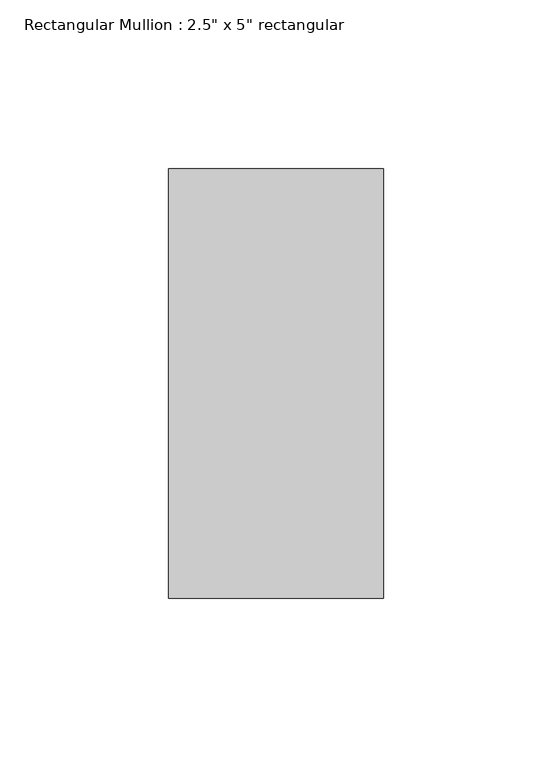
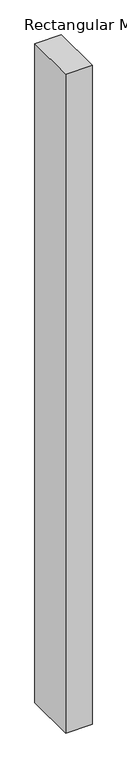
"""IFC4 building model written with IfcOpenShell, lengths in millimetres: member geometry."""

from ifc_helpers import new_model, si_unit, frame, origin, place, context, project, spatial, polyline, outline, extrude, source, transform, mapped, element, save


def member_562a4c76(model_context):
    return source(origin(), model_context, "Body", "SweptSolid", [
        extrude(outline(polyline([(0.0, 63.5), (0.0, -63.5), (-63.5, -63.5), (-63.5, 63.5), (0.0, 63.5)])), frame((0.0, 0.0, -1668.686135), z_axis=(0.0, 0.0, 1.0), x_axis=(1.0, 0.0, 0.0)), (0.0, 0.0, 1.0), 1668.686135),
    ])


if __name__ == "__main__":
    model = new_model("IFC4")
    model_context = context("Model", 3, world=origin())
    ifc_project = project(units=[si_unit("LENGTHUNIT", "METRE", prefix="MILLI")], contexts=[model_context])
    site = spatial("IfcSite", under=ifc_project)
    building = spatial("IfcBuilding", under=site)
    placement = place(None, origin())
    member_shape = member_562a4c76(model_context)
    element("IfcMember", 1, ObjectType="Rectangular Mullion : 2.5\" x 5\" rectangular", at=placement, inside=building, context=model_context, shape_type="MappedRepresentation", body=[
        mapped(member_shape, transform((0.0, 0.0, 0.0), x_axis=(1.0, 0.0, 0.0), y_axis=(0.0, 1.0, 0.0), z_axis=(0.0, 0.0, 1.0))),
    ])
    save(model, "model.ifc")

# Revit data of these elements
# Type "Rectangular Mullion : 2.5\" x 5\" rectangular"
#   built-in parameter 1007304 = 0.416667 (stored number, unit not read)
#   built-in parameter 1007301 = 0.104167 (stored number, unit not read)
#   built-in parameter 1007300 = 0.104167 (stored number, unit not read)
# Element 1 (IfcMember, "Rectangular Mullion : 2.5\" x 5\" rectangular")
#   Materials on its faces: "Aluminum"
# Materials
#   "Aluminum": class "Metal", colour RGB 247 247 247, transparency 0, Description = "Aluminum 6061", Cost = 0
